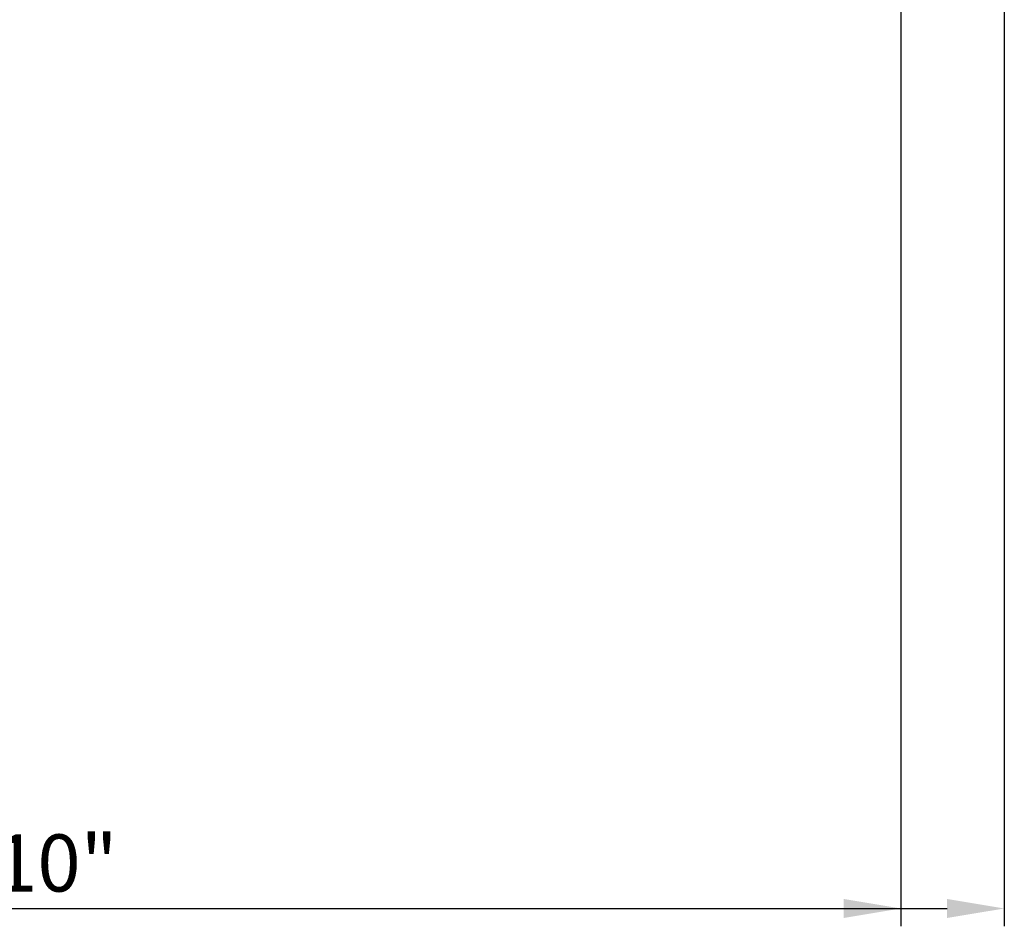
# Model space of a CAD drawing. Units: inches. Extents: x 2091 to 2899, y 967 to 2217.
# Tile 30 of 256: x 2390 to 2459, y 969 to 1033. Entities that reach past the tile are written whole.
import ezdxf

# ---------------------------------------------------------------- set-up
doc = ezdxf.new("R2010")
doc.units = ezdxf.units.IN
doc.layers.add('A-ANNO-DIMS', color=2, linetype='Continuous', lineweight=18)
doc.styles.get("Standard").update_dxf_attribs({"font": 'arial.ttf'})
doc.dimstyles.new('ISO-25', dxfattribs={"dimtxt": 4, "dimasz": 4, "dimexe": 1.25, "dimexo": 0.625, "dimtad": 1, "dimdec": 0, "dimlunit": 3, "dimtxsty": 'Standard', "dimcen": 2.5, "dimadec": 0, "dimazin": 0, "dimtfac": 1, "dimtdec": 0, "dimtmove": 0, "dimatfit": 3, "dimfxl": 1, "dimarcsym": 0})

# ---------------------------------------------------------------- blocks, each defined once
blk = doc.blocks.new('*D68')
at = {"layer": 'A-ANNO-DIMS', "color": 0, "lineweight": -2, "transparency": 16777216}
for p, q in [((2317.144, 1535.794), (2317.144, 969.464)), ((2459.384, 1535.794), (2459.384, 969.464)), ((2321.144, 970.714), (2455.384, 970.714))]:
    blk.add_line(p, q, dxfattribs=at)
at = {"layer": 'A-ANNO-DIMS', "color": 0, "transparency": 16777216}
for points in [[(2321.144, 971.381), (2321.144, 970.048), (2317.144, 970.714)], [(2455.384, 971.381), (2455.384, 970.048), (2459.384, 970.714)]]:
    blk.add_solid(points, dxfattribs=at)
at = {"layer": 'Defpoints', "color": 0, "transparency": 16777216}
for p in [(2317.144, 1536.419), (2459.384, 1536.419), (2459.384, 970.714)]:
    blk.add_point(p, dxfattribs=at)
at = {"layer": 'A-ANNO-DIMS', "color": 0, "transparency": 16777216, "insert": (2388.264, 973.382), "char_height": 4, "attachment_point": 5}
blk.add_mtext('11\'-10"', dxfattribs=at)
blk = doc.blocks.new('*D71')
at = {"layer": 'A-ANNO-DIMS', "color": 0, "lineweight": -2, "transparency": 16777216}
for p, q in [((2212.144, 1351.294), (2212.144, 969.464)), ((2452.144, 1351.294), (2452.144, 969.464)), ((2216.144, 970.714), (2448.144, 970.714))]:
    blk.add_line(p, q, dxfattribs=at)
at = {"layer": 'A-ANNO-DIMS', "color": 0, "transparency": 16777216}
for points in [[(2216.144, 971.381), (2216.144, 970.048), (2212.144, 970.714)], [(2448.144, 971.381), (2448.144, 970.048), (2452.144, 970.714)]]:
    blk.add_solid(points, dxfattribs=at)
at = {"layer": 'Defpoints', "color": 0, "transparency": 16777216}
for p in [(2212.144, 1351.919), (2452.144, 1351.919), (2452.144, 970.714)]:
    blk.add_point(p, dxfattribs=at)
at = {"layer": 'A-ANNO-DIMS', "color": 0, "transparency": 16777216, "insert": (2332.144, 973.382), "char_height": 4, "attachment_point": 5}
blk.add_mtext('20\'-0"', dxfattribs=at)

msp = doc.modelspace()

# ---------------------------------------------------------------- dimensions: what is measured, and where the dimension line sits
at = {"layer": 'A-ANNO-DIMS'}
for base, p1, p2, picture, middle in [((2459.384, 970.714), (2317.144, 1536.419), (2459.384, 1536.419), '*D68', (2388.264, 973.382)), ((2452.144, 970.714), (2212.144, 1351.919), (2452.144, 1351.919), '*D71', (2332.144, 973.382))]:
    dim = msp.add_linear_dim(base=base, p1=p1, p2=p2, dimstyle='ISO-25', override={"dimdec": 1, "dimlfac": 1, "dimrnd": 0, "dimzin": 1, "dimdsep": 46, "dimlunit": 4, "dimfrac": 2}, dxfattribs=at)
    dim.commit()
    dim.dimension.update_dxf_attribs({"geometry": picture, "text_midpoint": middle})

doc.saveas('drawing.dxf')
